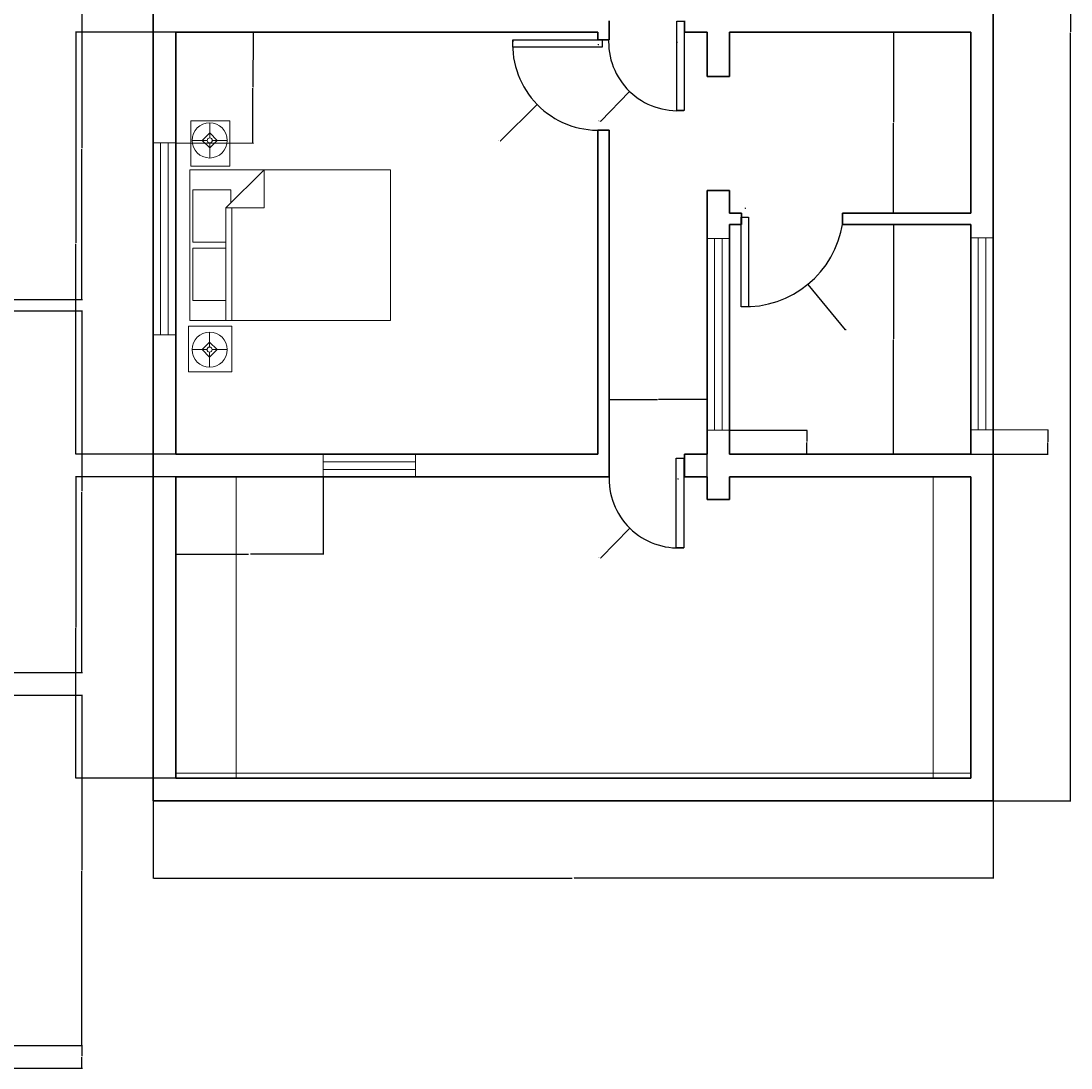
# Model space of a CAD drawing. Units: inches. Extents: x -52 to 1967, y 32 to 824.
# Tile 4 of 10: x 715 to 1133, y 68 to 485. Entities that reach past the tile are written whole.
import ezdxf

# ---------------------------------------------------------------- set-up
doc = ezdxf.new("R2010")
doc.units = ezdxf.units.IN
for name, color, linetype, lineweight in [('A-ANNO-DIMS', 2, 'Continuous', 18), ('A-DOOR', 3, 'Continuous', 25), ('A-FLOR', 7, 'Continuous', 18), ('A-FURN', 8, 'Continuous', 18), ('A-GLAZ', 4, 'Continuous', 18), ('A-WALL', 7, 'Continuous', 35)]:
    doc.layers.add(name, color=color, linetype=linetype, lineweight=lineweight)
doc.styles.get("Standard").update_dxf_attribs({"font": 'arial.ttf'})
doc.dimstyles.get("Standard").update_dxf_attribs({"dimtxt": 0.18, "dimasz": 0.18, "dimexe": 0.18, "dimexo": 0.0625, "dimgap": 0.09, "dimtad": 0, "dimtih": 1, "dimtoh": 1, "dimdec": 4, "dimzin": 0, "dimdsep": 46, "dimtxsty": 'Standard', "dimcen": 0.09, "dimadec": 0, "dimazin": 0, "dimtfac": 1, "dimtdec": 4, "dimtofl": 0, "dimtmove": 0, "dimatfit": 3, "dimfxl": 1, "dimtolj": 1, "dimtzin": 0, "dimarcsym": 0})

# ---------------------------------------------------------------- blocks, each defined once
blk = doc.blocks.new('WIN-WIDE-76IN')
for p, q in [((0, 0), (0, 9)), ((0, 9), (76.34, 9)), ((76.34, 9), (76.34, 0)), ((76.34, 6), (0, 6)), ((0, 3), (76.34, 3)), ((76.34, 0), (0, 0))]:
    blk.add_line(p, q)
blk = doc.blocks.new('WIN-NARROW-37IN')
for p, q in [((0, 0), (0, 9)), ((0, 9), (36.78, 9)), ((36.78, 0), (36.78, 9)), ((36.78, 6), (0, 6)), ((0, 3), (36.78, 3)), ((36.78, 0), (0, 0))]:
    blk.add_line(p, q)
blk = doc.blocks.new('DOOR-LEAF-36IN')
blk.add_lwpolyline([(0, 0), (-2.98, 0), (-2.98, 35.63), (0, 35.63)], close=True)
blk = doc.blocks.new('Bed - Queen')
for p, q in [((0, -80.00003), (0, 0)), ((0, 0), (59.99999, 0)), ((59.99999, 0), (59.99999, -80.00003)), ((7.99999, -1.2), (28.79998, -1.2)), ((7.99999, -14.4), (7.99999, -1.2)), ((28.79998, -1.2), (28.79998, -14.4)), ((31.19999, -1.2), (51.99999, -1.2)), ((31.19999, -14.4), (31.19999, -1.2)), ((51.99999, -1.2), (51.99999, -16.4)), ((0, -14.4), (44.8, -14.4)), ((59.99999, -29.6), (44.8, -14.4)), ((44.8, -14.4), (44.8, -29.6)), ((51.99999, -16.4), (46.79936, -16.4)), ((44.8, -16.8), (0, -16.8)), ((44.8, -29.6), (59.99999, -29.6)), ((59.99999, -80.00003), (0, -80.00003))]:
    blk.add_line(p, q)
blk = doc.blocks.new('Lamp - Table')
for p, q in [((0, 7), (0, 1)), ((-1, 0), (-7, 0)), ((0, 3), (-3, 0)), ((-3, 0), (0, -3)), ((3, 0), (0, 3)), ((0, -3), (3, 0)), ((1, 0), (7, 0)), ((0, -1), (0, -7))]:
    blk.add_line(p, q)
for radius in [7, 1]:
    blk.add_circle((0, 0), radius)
blk = doc.blocks.new('BED-QUEEN-WITH-NIGHTSTANDS')
for points in [[(0.4, 61.39), (15.92, 61.39), (15.92, 79.53), (0.4, 79.53)], [(-0.42, -2.26), (16.73, -2.26), (16.73, -20.45), (-0.42, -20.45)]]:
    blk.add_lwpolyline(points, close=True)
for p in [(7.97, 71.69), (7.93, -11.61)]:
    blk.add_blockref('Lamp - Table', p)
at = {"rotation": 90}
blk.add_blockref('Bed - Queen', (0, 0), dxfattribs=at)
blk = doc.blocks.new('*D66')
at = {"layer": 'A-ANNO-DIMS', "color": 0, "lineweight": -2, "transparency": 16777216}
for p, q in [((694.09, 493.97), (739.35, 493.97)), ((739.17, 493.79), (739.17, 434.16)), ((739.17, 374.15), (739.17, 433.79)), ((694.09, 373.97), (739.35, 373.97))]:
    blk.add_line(p, q, dxfattribs=at)
at = {"layer": 'A-ANNO-DIMS', "color": 0, "transparency": 16777216}
for points in [[(739.14, 493.79), (739.2, 493.79), (739.17, 493.97)], [(739.14, 374.15), (739.2, 374.15), (739.17, 373.97)]]:
    blk.add_solid(points, dxfattribs=at)
at = {"layer": 'Defpoints', "color": 0, "transparency": 16777216}
for p in [(694.03, 493.97), (739.17, 493.97), (694.03, 373.97)]:
    blk.add_point(p, dxfattribs=at)
at = {"layer": 'A-ANNO-DIMS', "color": 0, "transparency": 16777216, "insert": (739.17, 433.97), "char_height": 0.18, "attachment_point": 5}
blk.add_mtext('\\A1;120', dxfattribs=at)
blk = doc.blocks.new('*D67')
at = {"layer": 'A-ANNO-DIMS', "color": 0, "lineweight": -2, "transparency": 16777216}
for p, q in [((694.09, 369.47), (739.35, 369.47)), ((739.17, 369.29), (739.17, 297.65)), ((739.17, 225.65), (739.17, 297.29)), ((694.09, 225.47), (739.35, 225.47))]:
    blk.add_line(p, q, dxfattribs=at)
at = {"layer": 'A-ANNO-DIMS', "color": 0, "transparency": 16777216}
for points in [[(739.14, 369.29), (739.2, 369.29), (739.17, 369.47)], [(739.14, 225.65), (739.2, 225.65), (739.17, 225.47)]]:
    blk.add_solid(points, dxfattribs=at)
at = {"layer": 'Defpoints', "color": 0, "transparency": 16777216}
for p in [(694.03, 369.47), (739.17, 369.47), (694.03, 225.47)]:
    blk.add_point(p, dxfattribs=at)
at = {"layer": 'A-ANNO-DIMS', "color": 0, "transparency": 16777216, "insert": (739.17, 297.47), "char_height": 0.18, "attachment_point": 5}
blk.add_mtext('\\A1;144', dxfattribs=at)
blk = doc.blocks.new('*D68')
at = {"layer": 'A-ANNO-DIMS', "color": 0, "lineweight": -2, "transparency": 16777216}
for p, q in [((694.09, 216.47), (739.35, 216.47)), ((739.17, 216.29), (739.17, 146.91)), ((739.17, 77.15), (739.17, 146.54)), ((694.09, 76.97), (739.35, 76.97))]:
    blk.add_line(p, q, dxfattribs=at)
at = {"layer": 'A-ANNO-DIMS', "color": 0, "transparency": 16777216}
for points in [[(739.14, 216.29), (739.2, 216.29), (739.17, 216.47)], [(739.14, 77.15), (739.2, 77.15), (739.17, 76.97)]]:
    blk.add_solid(points, dxfattribs=at)
at = {"layer": 'Defpoints', "color": 0, "transparency": 16777216}
for p in [(694.03, 216.47), (739.17, 216.47), (694.03, 76.97)]:
    blk.add_point(p, dxfattribs=at)
at = {"layer": 'A-ANNO-DIMS', "color": 0, "transparency": 16777216, "insert": (739.17, 146.72), "char_height": 0.18, "attachment_point": 5}
blk.add_mtext('\\A1;139.5', dxfattribs=at)
blk = doc.blocks.new('*D69')
at = {"layer": 'A-ANNO-DIMS', "color": 0, "lineweight": -2, "transparency": 16777216}
for p, q in [((694.09, 76.97), (739.35, 76.97)), ((739.17, 76.79), (739.17, 72.66)), ((739.17, 68.15), (739.17, 72.29)), ((703.09, 67.97), (739.35, 67.97))]:
    blk.add_line(p, q, dxfattribs=at)
at = {"layer": 'A-ANNO-DIMS', "color": 0, "transparency": 16777216}
for points in [[(739.14, 76.79), (739.2, 76.79), (739.17, 76.97)], [(739.14, 68.15), (739.2, 68.15), (739.17, 67.97)]]:
    blk.add_solid(points, dxfattribs=at)
at = {"layer": 'Defpoints', "color": 0, "transparency": 16777216}
for p in [(694.03, 76.97), (739.17, 76.97), (703.03, 67.97)]:
    blk.add_point(p, dxfattribs=at)
at = {"layer": 'A-ANNO-DIMS', "color": 0, "transparency": 16777216, "insert": (739.17, 72.47), "char_height": 0.18, "attachment_point": 5}
blk.add_mtext('\\A1;9', dxfattribs=at)
blk = doc.blocks.new('*D93')
at = {"layer": 'A-ANNO-DIMS', "color": 0, "lineweight": -2, "transparency": 16777216}
for p, q in [((767.57, 174.29), (767.57, 143.44)), ((1102.07, 174.29), (1102.07, 143.44)), ((767.75, 143.62), (934.42, 143.62)), ((1101.89, 143.62), (935.21, 143.62))]:
    blk.add_line(p, q, dxfattribs=at)
at = {"layer": 'A-ANNO-DIMS', "color": 0, "transparency": 16777216}
for points in [[(767.75, 143.65), (767.75, 143.59), (767.57, 143.62)], [(1101.89, 143.65), (1101.89, 143.59), (1102.07, 143.62)]]:
    blk.add_solid(points, dxfattribs=at)
at = {"layer": 'Defpoints', "color": 0, "transparency": 16777216}
for p in [(767.57, 174.35), (1102.07, 174.35), (1102.07, 143.62)]:
    blk.add_point(p, dxfattribs=at)
at = {"layer": 'A-ANNO-DIMS', "color": 0, "transparency": 16777216, "insert": (934.82, 143.62), "char_height": 0.18, "attachment_point": 5}
blk.add_mtext('\\A1;334.5', dxfattribs=at)
blk = doc.blocks.new('*D94')
at = {"layer": 'A-ANNO-DIMS', "color": 0, "lineweight": -2, "transparency": 16777216}
for p, q in [((1102.13, 786.35), (1132.97, 786.35)), ((1132.79, 786.17), (1132.79, 480.53)), ((1132.79, 174.53), (1132.79, 480.17)), ((1102.13, 174.35), (1132.97, 174.35))]:
    blk.add_line(p, q, dxfattribs=at)
at = {"layer": 'A-ANNO-DIMS', "color": 0, "transparency": 16777216}
for points in [[(1132.76, 786.17), (1132.82, 786.17), (1132.79, 786.35)], [(1132.76, 174.53), (1132.82, 174.53), (1132.79, 174.35)]]:
    blk.add_solid(points, dxfattribs=at)
at = {"layer": 'Defpoints', "color": 0, "transparency": 16777216}
for p in [(1102.07, 786.35), (1132.79, 786.35), (1102.07, 174.35)]:
    blk.add_point(p, dxfattribs=at)
at = {"layer": 'A-ANNO-DIMS', "color": 0, "transparency": 16777216, "insert": (1132.79, 480.35), "char_height": 0.18, "attachment_point": 5}
blk.add_mtext('\\A1;612', dxfattribs=at)
blk = doc.blocks.new('*D102')
at = {"layer": 'A-ANNO-DIMS', "color": 0, "lineweight": -2, "transparency": 16777216}
for p, q in [((1093.01, 480.35), (1062.16, 480.35)), ((1062.34, 480.17), (1062.34, 444.53)), ((1062.34, 408.53), (1062.34, 444.17)), ((1093.01, 408.35), (1062.16, 408.35))]:
    blk.add_line(p, q, dxfattribs=at)
at = {"layer": 'A-ANNO-DIMS', "color": 0, "transparency": 16777216}
for points in [[(1062.31, 480.17), (1062.37, 480.17), (1062.34, 480.35)], [(1062.31, 408.53), (1062.37, 408.53), (1062.34, 408.35)]]:
    blk.add_solid(points, dxfattribs=at)
at = {"layer": 'Defpoints', "color": 0, "transparency": 16777216}
for p in [(1062.34, 480.35), (1093.07, 480.35), (1093.07, 408.35)]:
    blk.add_point(p, dxfattribs=at)
at = {"layer": 'A-ANNO-DIMS', "color": 0, "transparency": 16777216, "insert": (1062.34, 444.35), "char_height": 0.18, "attachment_point": 5}
blk.add_mtext('\\A1;72', dxfattribs=at)
blk = doc.blocks.new('*D103')
at = {"layer": 'A-ANNO-DIMS', "color": 0, "lineweight": -2, "transparency": 16777216}
for p, q in [((1093.01, 403.85), (1062.16, 403.85)), ((1062.34, 403.67), (1062.34, 358.28)), ((1062.34, 312.53), (1062.34, 357.92)), ((1093.01, 312.35), (1062.16, 312.35))]:
    blk.add_line(p, q, dxfattribs=at)
at = {"layer": 'A-ANNO-DIMS', "color": 0, "transparency": 16777216}
for points in [[(1062.31, 403.67), (1062.37, 403.67), (1062.34, 403.85)], [(1062.31, 312.53), (1062.37, 312.53), (1062.34, 312.35)]]:
    blk.add_solid(points, dxfattribs=at)
at = {"layer": 'Defpoints', "color": 0, "transparency": 16777216}
for p in [(1062.34, 403.85), (1093.07, 403.85), (1093.07, 312.35)]:
    blk.add_point(p, dxfattribs=at)
at = {"layer": 'A-ANNO-DIMS', "color": 0, "transparency": 16777216, "insert": (1062.34, 358.1), "char_height": 0.18, "attachment_point": 5}
blk.add_mtext('\\A1;91.5', dxfattribs=at)
blk = doc.blocks.new('*D104')
at = {"layer": 'A-ANNO-DIMS', "color": 0, "lineweight": -2, "transparency": 16777216}
for p, q in [((776.51, 480.35), (736.6, 480.35)), ((736.78, 480.17), (736.78, 396.53)), ((736.78, 312.53), (736.78, 396.17)), ((776.51, 312.35), (736.6, 312.35))]:
    blk.add_line(p, q, dxfattribs=at)
at = {"layer": 'A-ANNO-DIMS', "color": 0, "transparency": 16777216}
for points in [[(736.75, 480.17), (736.81, 480.17), (736.78, 480.35)], [(736.75, 312.53), (736.81, 312.53), (736.78, 312.35)]]:
    blk.add_solid(points, dxfattribs=at)
at = {"layer": 'Defpoints', "color": 0, "transparency": 16777216}
for p in [(736.78, 480.35), (776.57, 480.35), (776.57, 312.35)]:
    blk.add_point(p, dxfattribs=at)
at = {"layer": 'A-ANNO-DIMS', "color": 0, "transparency": 16777216, "insert": (736.78, 396.35), "char_height": 0.18, "attachment_point": 5}
blk.add_mtext('\\A1;168', dxfattribs=at)
blk = doc.blocks.new('*D106')
at = {"layer": 'A-ANNO-DIMS', "color": 0, "lineweight": -2, "transparency": 16777216}
for p, q in [((776.51, 303.35), (736.6, 303.35)), ((736.78, 303.17), (736.78, 243.53)), ((736.78, 183.53), (736.78, 243.17)), ((776.51, 183.35), (736.6, 183.35))]:
    blk.add_line(p, q, dxfattribs=at)
at = {"layer": 'A-ANNO-DIMS', "color": 0, "transparency": 16777216}
for points in [[(736.75, 303.17), (736.81, 303.17), (736.78, 303.35)], [(736.75, 183.53), (736.81, 183.53), (736.78, 183.35)]]:
    blk.add_solid(points, dxfattribs=at)
at = {"layer": 'Defpoints', "color": 0, "transparency": 16777216}
for p in [(736.78, 303.35), (776.57, 303.35), (776.57, 183.35)]:
    blk.add_point(p, dxfattribs=at)
at = {"layer": 'A-ANNO-DIMS', "color": 0, "transparency": 16777216, "insert": (736.78, 243.35), "char_height": 0.18, "attachment_point": 5}
blk.add_mtext('\\A1;120', dxfattribs=at)
blk = doc.blocks.new('*D110')
at = {"layer": 'A-ANNO-DIMS', "color": 0, "lineweight": -2, "transparency": 16777216}
for p, q in [((776.57, 303.29), (776.53, 272.44)), ((835.19, 303.22), (835.16, 272.38)), ((776.71, 272.62), (805.45, 272.59)), ((834.98, 272.56), (806.24, 272.59))]:
    blk.add_line(p, q, dxfattribs=at)
at = {"layer": 'A-ANNO-DIMS', "color": 0, "transparency": 16777216}
for points in [[(776.71, 272.65), (776.71, 272.59), (776.53, 272.62)], [(834.98, 272.59), (834.98, 272.53), (835.16, 272.56)]]:
    blk.add_solid(points, dxfattribs=at)
at = {"layer": 'Defpoints', "color": 0, "transparency": 16777216}
for p in [(776.57, 303.35), (835.19, 303.28), (776.53, 272.62)]:
    blk.add_point(p, dxfattribs=at)
at = {"layer": 'A-ANNO-DIMS', "color": 0, "transparency": 16777216, "insert": (805.85, 272.59), "char_height": 0.18, "attachment_point": 5}
blk.add_mtext('\\A1;58.62', dxfattribs=at)
blk = doc.blocks.new('*D111')
at = {"layer": 'A-ANNO-DIMS', "color": 0, "lineweight": -2, "transparency": 16777216}
for p, q in [((949.07, 303.41), (949.07, 334.25)), ((949.25, 334.07), (968.35, 334.07)), ((987.89, 334.07), (968.79, 334.07)), ((988.07, 303.41), (988.07, 334.25))]:
    blk.add_line(p, q, dxfattribs=at)
at = {"layer": 'A-ANNO-DIMS', "color": 0, "transparency": 16777216}
for points in [[(949.25, 334.1), (949.25, 334.04), (949.07, 334.07)], [(987.89, 334.1), (987.89, 334.04), (988.07, 334.07)]]:
    blk.add_solid(points, dxfattribs=at)
at = {"layer": 'Defpoints', "color": 0, "transparency": 16777216}
for p in [(988.07, 334.07), (949.07, 303.35), (988.07, 303.35)]:
    blk.add_point(p, dxfattribs=at)
at = {"layer": 'A-ANNO-DIMS', "color": 0, "transparency": 16777216, "insert": (968.57, 334.07), "char_height": 0.18, "attachment_point": 5}
blk.add_mtext('\\A1;39', dxfattribs=at)
blk = doc.blocks.new('*D114')
at = {"layer": 'A-ANNO-DIMS', "color": 0, "lineweight": -2, "transparency": 16777216}
for p, q in [((776.63, 480.35), (807.47, 480.3)), ((807.29, 480.12), (807.26, 458.45)), ((807.23, 436.42), (807.26, 458.09)), ((776.57, 436.28), (807.41, 436.24))]:
    blk.add_line(p, q, dxfattribs=at)
at = {"layer": 'A-ANNO-DIMS', "color": 0, "transparency": 16777216}
for points in [[(807.26, 480.12), (807.32, 480.12), (807.29, 480.3)], [(807.2, 436.42), (807.26, 436.42), (807.23, 436.24)]]:
    blk.add_solid(points, dxfattribs=at)
at = {"layer": 'Defpoints', "color": 0, "transparency": 16777216}
for p in [(776.57, 480.35), (776.5, 436.28), (807.23, 436.24)]:
    blk.add_point(p, dxfattribs=at)
at = {"layer": 'A-ANNO-DIMS', "color": 0, "transparency": 16777216, "insert": (807.26, 458.27), "char_height": 0.18, "attachment_point": 5}
blk.add_mtext('\\A1;44.07', dxfattribs=at)
blk = doc.blocks.new('*D116')
at = {"layer": 'A-ANNO-DIMS', "color": 0, "lineweight": -2, "transparency": 16777216}
for p, q in [((997.12, 321.88), (1027.96, 321.93)), ((1027.78, 321.75), (1027.79, 317.35)), ((1027.79, 312.58), (1027.79, 316.98)), ((997.13, 312.35), (1027.97, 312.4))]:
    blk.add_line(p, q, dxfattribs=at)
at = {"layer": 'A-ANNO-DIMS', "color": 0, "transparency": 16777216}
for points in [[(1027.81, 321.75), (1027.75, 321.75), (1027.78, 321.93)], [(1027.82, 312.58), (1027.76, 312.58), (1027.79, 312.4)]]:
    blk.add_solid(points, dxfattribs=at)
at = {"layer": 'Defpoints', "color": 0, "transparency": 16777216}
for p in [(997.05, 321.88), (997.07, 312.35), (1027.79, 312.4)]:
    blk.add_point(p, dxfattribs=at)
at = {"layer": 'A-ANNO-DIMS', "color": 0, "transparency": 16777216, "insert": (1027.79, 317.17), "char_height": 0.18, "attachment_point": 5}
blk.add_mtext('\\A1;9.535', dxfattribs=at)
blk = doc.blocks.new('*D118')
at = {"layer": 'A-ANNO-DIMS', "color": 0, "lineweight": -2, "transparency": 16777216}
for p, q in [((1093.12, 322.12), (1123.96, 322.15)), ((1123.78, 321.97), (1123.79, 317.45)), ((1123.79, 312.56), (1123.79, 317.08)), ((1093.13, 312.35), (1123.97, 312.38))]:
    blk.add_line(p, q, dxfattribs=at)
at = {"layer": 'A-ANNO-DIMS', "color": 0, "transparency": 16777216}
for points in [[(1123.81, 321.97), (1123.75, 321.97), (1123.78, 322.15)], [(1123.82, 312.56), (1123.76, 312.56), (1123.79, 312.38)]]:
    blk.add_solid(points, dxfattribs=at)
at = {"layer": 'Defpoints', "color": 0, "transparency": 16777216}
for p in [(1093.06, 322.12), (1093.07, 312.35), (1123.79, 312.38)]:
    blk.add_point(p, dxfattribs=at)
at = {"layer": 'A-ANNO-DIMS', "color": 0, "transparency": 16777216, "insert": (1123.79, 317.27), "char_height": 0.18, "attachment_point": 5}
blk.add_mtext('\\A1;9.775', dxfattribs=at)
blk = doc.blocks.new('*D141')
at = {"layer": 'A-ANNO-DIMS', "color": 0, "lineweight": -2, "transparency": 16777216}
for p, q in [((1003.24, 410.31), (1003.42, 410.31)), ((1003.33, 410.22), (1003.33, 410.4)), ((1043.23, 361.85), (1028.38, 379.88)), ((1043.41, 361.85), (1043.23, 361.85))]:
    blk.add_line(p, q, dxfattribs=at)
at = {"layer": 'A-ANNO-DIMS', "color": 0, "transparency": 16777216}
blk.add_solid([(1028.41, 379.9), (1028.36, 379.86), (1028.27, 380.02)], dxfattribs=at)
at = {"layer": 'Defpoints', "color": 0, "transparency": 16777216}
for p in [(1003.33, 410.31), (1028.27, 380.02)]:
    blk.add_point(p, dxfattribs=at)
at = {"layer": 'A-ANNO-DIMS', "color": 0, "transparency": 16777216, "insert": (1043.96, 361.85), "char_height": 0.18, "attachment_point": 5}
blk.add_mtext('\\A1;R39.234', dxfattribs=at)
blk = doc.blocks.new('*D144')
at = {"layer": 'A-ANNO-DIMS', "color": 0, "lineweight": -2, "transparency": 16777216}
for p, q in [((944.7, 475.47), (944.88, 475.47)), ((944.79, 475.38), (944.79, 475.56)), ((905.85, 437.18), (920.32, 451.41)), ((905.67, 437.18), (905.85, 437.18))]:
    blk.add_line(p, q, dxfattribs=at)
at = {"layer": 'A-ANNO-DIMS', "color": 0, "transparency": 16777216}
blk.add_solid([(920.3, 451.44), (920.34, 451.39), (920.45, 451.54)], dxfattribs=at)
at = {"layer": 'Defpoints', "color": 0, "transparency": 16777216}
for p in [(944.79, 475.47), (920.45, 451.54)]:
    blk.add_point(p, dxfattribs=at)
at = {"layer": 'A-ANNO-DIMS', "color": 0, "transparency": 16777216, "insert": (905.19, 437.18), "char_height": 0.18, "attachment_point": 5}
blk.add_mtext('\\A1;R34.13', dxfattribs=at)
blk = doc.blocks.new('*D145')
at = {"layer": 'A-ANNO-DIMS', "color": 0, "lineweight": -2, "transparency": 16777216}
for p, q in [((976.47, 302.57), (976.65, 302.57)), ((976.56, 302.48), (976.56, 302.66)), ((945.78, 271.08), (957.2, 282.76)), ((945.6, 271.08), (945.78, 271.08))]:
    blk.add_line(p, q, dxfattribs=at)
at = {"layer": 'A-ANNO-DIMS', "color": 0, "transparency": 16777216}
blk.add_solid([(957.18, 282.78), (957.22, 282.74), (957.32, 282.89)], dxfattribs=at)
at = {"layer": 'Defpoints', "color": 0, "transparency": 16777216}
for p in [(976.56, 302.57), (957.32, 282.89)]:
    blk.add_point(p, dxfattribs=at)
at = {"layer": 'A-ANNO-DIMS', "color": 0, "transparency": 16777216, "insert": (945.05, 271.08), "char_height": 0.18, "attachment_point": 5}
blk.add_mtext('\\A1;R27.525', dxfattribs=at)
blk = doc.blocks.new('*D146')
at = {"layer": 'A-ANNO-DIMS', "color": 0, "lineweight": -2, "transparency": 16777216}
for p, q in [((976.14, 476.47), (976.32, 476.47)), ((976.23, 476.38), (976.23, 476.56)), ((945.83, 445.01), (957.11, 456.68)), ((945.65, 445.01), (945.83, 445.01))]:
    blk.add_line(p, q, dxfattribs=at)
at = {"layer": 'A-ANNO-DIMS', "color": 0, "transparency": 16777216}
blk.add_solid([(957.09, 456.7), (957.13, 456.66), (957.23, 456.81)], dxfattribs=at)
at = {"layer": 'Defpoints', "color": 0, "transparency": 16777216}
for p in [(976.23, 476.47), (957.23, 456.81)]:
    blk.add_point(p, dxfattribs=at)
at = {"layer": 'A-ANNO-DIMS', "color": 0, "transparency": 16777216, "insert": (945.1, 445.01), "char_height": 0.18, "attachment_point": 5}
blk.add_mtext('\\A1;R27.343', dxfattribs=at)

msp = doc.modelspace()

# ---------------------------------------------------------------- linework, layer by layer
at = {"layer": 'A-DOOR'}
for centre, radius, start, end in [((944.7861, 475.4699), 34.1317, 176.874954, 272.157751), ((976.2328, 476.4706), 27.343, 176.379178, 275.582062), ((1003.3331, 410.3113), 39.2341, 267.498399, 351.423572), ((976.563, 302.5748), 27.5251, 176.685191, 274.62366)]:
    msp.add_arc(centre, radius, start, end, dxfattribs=at)
at = {"layer": 'A-FLOR'}
for p, q in [((800.5687, 183.3484), (800.5687, 303.3484)), ((1078.0687, 183.3484), (1078.0687, 303.3484)), ((776.5687, 185.3484), (1093.0687, 185.3484))]:
    msp.add_line(p, q, dxfattribs=at)
at = {"layer": 'A-WALL'}
for p, q in [((767.5687, 174.3484), (767.5687, 786.3484)), ((1102.0687, 174.3484), (1102.0687, 786.3484)), ((949.0687, 477.3484), (949.0687, 484.8484)), ((979.0687, 480.3484), (979.0687, 484.8484)), ((776.5687, 480.3484), (944.5687, 480.3484)), ((776.5687, 312.3484), (776.5687, 480.3484)), ((944.5687, 477.3484), (944.5687, 480.3484)), ((944.5687, 477.3484), (949.0687, 477.3484)), ((979.0687, 480.3484), (988.0687, 480.3484)), ((988.0687, 462.6874), (988.0687, 480.3484)), ((997.0687, 462.6874), (997.0687, 480.3484)), ((997.0687, 480.3484), (1093.0687, 480.3484)), ((1093.0687, 408.3484), (1093.0687, 480.3484)), ((988.0687, 462.6874), (997.0687, 462.6874)), ((944.5687, 312.3484), (944.5687, 441.3484)), ((944.5687, 441.3484), (949.0687, 441.3484)), ((949.0687, 303.3484), (949.0687, 441.3484)), ((988.0687, 417.3484), (997.0687, 417.3484)), ((988.0687, 312.3484), (988.0687, 417.3484)), ((997.0687, 408.3484), (997.0687, 417.3484)), ((997.0687, 408.3484), (1001.7298, 408.3484)), ((1001.7298, 403.8484), (1001.7298, 408.3484)), ((1042.0687, 403.8484), (1042.0687, 408.3484)), ((1042.0687, 408.3484), (1093.0687, 408.3484)), ((997.0687, 403.8484), (1001.7298, 403.8484)), ((997.0687, 312.3484), (997.0687, 403.8484)), ((1042.0687, 403.8484), (1093.0687, 403.8484)), ((1093.0687, 312.3484), (1093.0687, 403.8484)), ((776.5687, 312.3484), (944.5687, 312.3484)), ((979.0687, 303.3484), (979.0687, 312.3484)), ((979.0687, 312.3484), (988.0687, 312.3484)), ((997.0687, 312.3484), (1093.0687, 312.3484)), ((776.5687, 303.3484), (949.0687, 303.3484)), ((776.5687, 183.3484), (776.5687, 303.3484)), ((979.0687, 303.3484), (988.0687, 303.3484)), ((988.0687, 294.3484), (988.0687, 303.3484)), ((997.0687, 294.3484), (997.0687, 303.3484)), ((997.0687, 303.3484), (1093.0687, 303.3484)), ((1093.0687, 183.3484), (1093.0687, 303.3484)), ((988.0687, 294.3484), (997.0687, 294.3484)), ((776.5687, 183.3484), (1093.0687, 183.3484)), ((767.5687, 174.3484), (1102.0687, 174.3484))]:
    msp.add_line(p, q, dxfattribs=at)

# ---------------------------------------------------------------- block references
at = {"layer": 'A-DOOR'}
for p in [(979.0057, 449.1942), (1004.5889, 371.0966), (978.798, 275.109)]:
    msp.add_blockref('DOOR-LEAF-36IN', p, dxfattribs=at)
at = {"layer": 'A-DOOR', "rotation": 269.9999999999999}
msp.add_blockref('DOOR-LEAF-36IN', (910.6878, 474.3722), dxfattribs=at)
at = {"layer": 'A-FURN'}
msp.add_blockref('BED-QUEEN-WITH-NIGHTSTANDS', (782.0737, 365.5948), dxfattribs=at)
at = {"layer": 'A-GLAZ'}
for p, rotation in [((767.5042, 436.281), 270), ((988.0532, 398.2236), 269.9999999999997), ((1093.0594, 398.4634), 270)]:
    msp.add_blockref('WIN-WIDE-76IN', p, dxfattribs=dict(at, rotation=rotation))
msp.add_blockref('WIN-NARROW-37IN', (835.1907, 303.2834), dxfattribs=at)

# ---------------------------------------------------------------- dimensions: what is measured, and where the dimension line sits
at = {"layer": 'A-ANNO-DIMS'}
for base, p1, p2, angle, override, picture, middle in [((1132.7937, 786.3484), (1102.0687, 174.3484), (1102.0687, 786.3484), 90, {"dimdec": 0, "dimlfac": 1, "dimrnd": 0, "dimzin": 0, "dimdsep": 46, "dimlunit": 2}, '*D94', (1132.7937, 480.3484)), ((739.1728, 493.9731), (694.0273, 373.9731), (694.0273, 493.9731), 90, {"dimdec": 0, "dimlfac": 1, "dimrnd": 0, "dimzin": 0, "dimdsep": 46, "dimlunit": 2}, '*D66', (739.1728, 433.9731)), ((736.7792, 480.3484), (776.5687, 312.3484), (776.5687, 480.3484), 90, {"dimdec": 0, "dimlfac": 1, "dimrnd": 0, "dimzin": 0, "dimdsep": 46, "dimlunit": 2}, '*D104', (736.7792, 396.3484)), ((807.2292, 436.2361), (776.5687, 480.3484), (776.5042, 436.281), 269.916117, {"dimdec": 2, "dimlfac": 1, "dimrnd": 0, "dimzin": 0, "dimdsep": 46, "dimlunit": 2}, '*D114', (807.2614, 458.2698)), ((1062.3437, 480.3484), (1093.0687, 408.3484), (1093.0687, 480.3484), 90, {"dimdec": 0, "dimlfac": 1, "dimrnd": 0, "dimzin": 0, "dimdsep": 46, "dimlunit": 2}, '*D102', (1062.3437, 444.3484)), ((1062.3437, 403.8484), (1093.0687, 312.3484), (1093.0687, 403.8484), 90, {"dimdec": 1, "dimlfac": 1, "dimrnd": 0, "dimzin": 0, "dimdsep": 46, "dimlunit": 2}, '*D103', (1062.3437, 358.0984)), ((739.1728, 369.4731), (694.0273, 225.4731), (694.0273, 369.4731), 90, {"dimdec": 0, "dimlfac": 1, "dimrnd": 0, "dimzin": 0, "dimdsep": 46, "dimlunit": 2}, '*D67', (739.1728, 297.4731)), ((1123.7937, 312.3777), (1093.0594, 322.1232), (1093.0687, 312.3484), 270.054651, {"dimdec": 3, "dimlfac": 1, "dimrnd": 0, "dimzin": 0, "dimdsep": 46, "dimlunit": 2}, '*D118', (1123.789, 317.2651)), ((1027.7937, 312.3985), (997.0532, 321.8835), (997.0687, 312.3484), 270.093347, {"dimdec": 3, "dimlfac": 1, "dimrnd": 0, "dimzin": 0, "dimdsep": 46, "dimlunit": 2}, '*D116', (1027.7859, 317.166)), ((736.7792, 303.3484), (776.5687, 183.3484), (776.5687, 303.3484), 90, {"dimdec": 0, "dimlfac": 1, "dimrnd": 0, "dimzin": 0, "dimdsep": 46, "dimlunit": 2}, '*D106', (736.7792, 243.3484)), ((776.5346, 272.6235), (835.1907, 303.2834), (776.5687, 303.3484), 179.936465, {"dimdec": 2, "dimlfac": 1, "dimrnd": 0, "dimzin": 0, "dimdsep": 46, "dimlunit": 2}, '*D110', (805.8456, 272.5909)), ((739.1728, 216.4731), (694.0273, 76.9731), (694.0273, 216.4731), 90, {"dimdec": 1, "dimlfac": 1, "dimrnd": 0, "dimzin": 0, "dimdsep": 46, "dimlunit": 2}, '*D68', (739.1728, 146.7231)), ((739.1728, 76.9731), (703.0273, 67.9731), (694.0273, 76.9731), 90, {"dimdec": 0, "dimlfac": 1, "dimrnd": 0, "dimzin": 0, "dimdsep": 46, "dimlunit": 2}, '*D69', (739.1728, 72.4731))]:
    dim = msp.add_linear_dim(base=base, p1=p1, p2=p2, angle=angle, dimstyle='Standard', override=override, dxfattribs=at)
    dim.commit()
    dim.dimension.update_dxf_attribs({"geometry": picture, "text_midpoint": middle})
for center, mpoint, override, picture, middle in [((944.7861, 475.4699), (920.4481, 451.5401), {"dimdec": 2, "dimlfac": 1, "dimrnd": 0, "dimzin": 0, "dimdsep": 46, "dimlunit": 2}, '*D144', (905.1854, 437.1822)), ((976.2328, 476.4706), (957.2321, 456.8081), {"dimdec": 3, "dimlfac": 1, "dimrnd": 0, "dimzin": 0, "dimdsep": 46, "dimlunit": 2}, '*D146', (945.1019, 445.0106)), ((1003.3331, 410.3113), (1028.2687, 380.0204), {"dimdec": 3, "dimlfac": 1, "dimrnd": 0, "dimzin": 0, "dimdsep": 46, "dimlunit": 2}, '*D141', (1043.9594, 361.8459)), ((976.563, 302.5748), (957.323, 282.891), {"dimdec": 3, "dimlfac": 1, "dimrnd": 0, "dimzin": 0, "dimdsep": 46, "dimlunit": 2}, '*D145', (945.0486, 271.0807))]:
    dim = msp.add_radius_dim(center=center, mpoint=mpoint, dimstyle='Standard', override=override, dxfattribs=at)
    dim.commit()
    dim.dimension.update_dxf_attribs({"geometry": picture, "text_midpoint": middle, "dimtype": 164})
for base, p1, p2, override, picture, middle in [((988.0687, 334.0734), (949.0687, 303.3484), (988.0687, 303.3484), {"dimdec": 0, "dimlfac": 1, "dimrnd": 0, "dimzin": 0, "dimdsep": 46, "dimlunit": 2}, '*D111', (968.5687, 334.0734)), ((1102.0687, 143.6234), (767.5687, 174.3484), (1102.0687, 174.3484), {"dimdec": 1, "dimlfac": 1, "dimrnd": 0, "dimzin": 0, "dimdsep": 46, "dimlunit": 2}, '*D93', (934.8187, 143.6234))]:
    dim = msp.add_linear_dim(base=base, p1=p1, p2=p2, dimstyle='Standard', override=override, dxfattribs=at)
    dim.commit()
    dim.dimension.update_dxf_attribs({"geometry": picture, "text_midpoint": middle})

doc.saveas('drawing.dxf')
